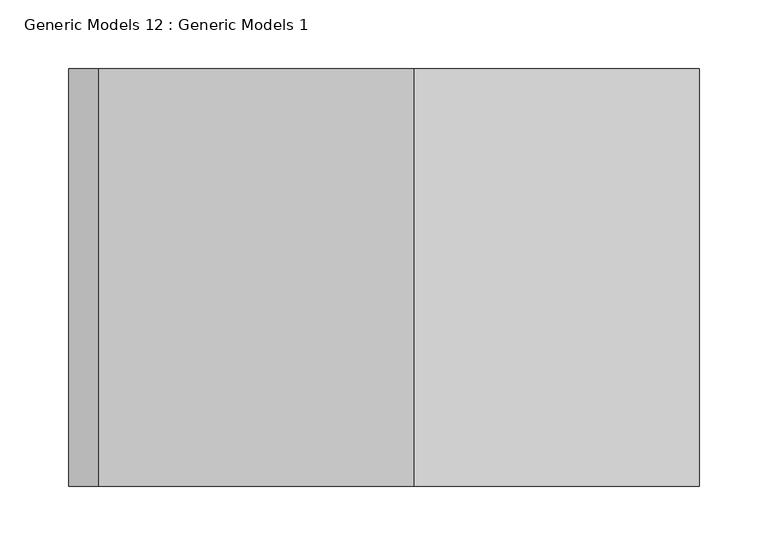
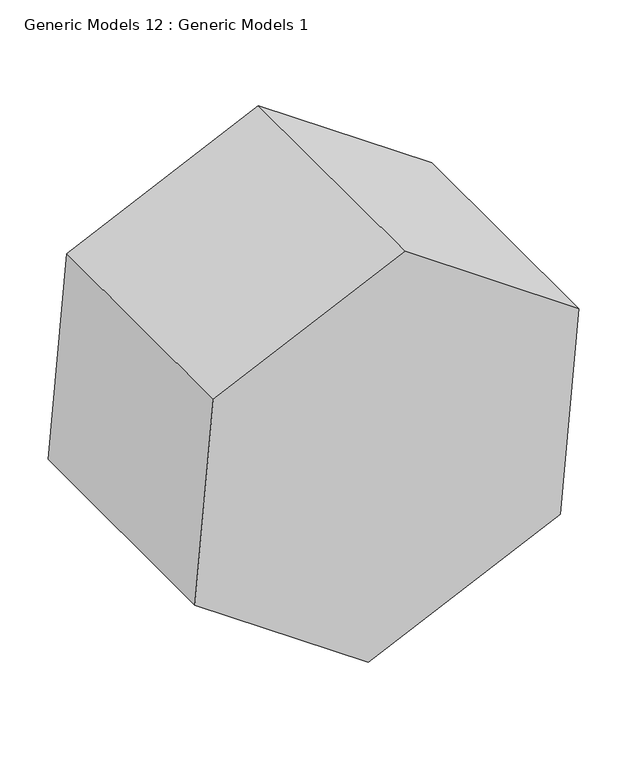
"""IFC4 building model written with IfcOpenShell, lengths in millimetres: proxy geometry, Generic Models 12 : Generic Models 1."""

from ifc_helpers import new_model, si_unit, frame, origin, place, context, project, spatial, polyline, outline, extrude, source, transform, mapped, element, save


def generic_models_12_generic_models_1_297bb3a6(model_context):
    return source(origin(), model_context, "Body", "SweptSolid", [
        extrude(outline(polyline([(833.1013393, 3247.6920945), (978.7897542, 3039.6274753), (871.4447157, 2809.4252974), (618.4112624, 2787.2877387), (472.7228475, 2995.352358), (580.067886, 3225.5545359), (833.1013393, 3247.6920945)])), frame((0.0, -10720.3372434, 0.0), z_axis=(0.0, 1.0, 0.0), x_axis=(0.0, 0.0, 1.0)), (0.0, 0.0, 1.0), 304.8),
    ])


if __name__ == "__main__":
    model = new_model("IFC4")
    model_context = context("Model", 3, world=origin())
    ifc_project = project(units=[si_unit("LENGTHUNIT", "METRE", prefix="MILLI")], contexts=[model_context])
    site = spatial("IfcSite", under=ifc_project)
    building = spatial("IfcBuilding", under=site)
    placement = place(None, origin())
    generic_models_12_generic_models_1_shape = generic_models_12_generic_models_1_297bb3a6(model_context)
    element("IfcBuildingElementProxy", 1, Name="Generic Models 12 : Generic Models 1", ObjectType="Generic Models 12 : Generic Models 1", at=placement, inside=building, context=model_context, shape_type="MappedRepresentation", body=[
        mapped(generic_models_12_generic_models_1_shape, transform((0.0, 0.0, 0.0), x_axis=(1.0, 0.0, 0.0), y_axis=(0.0, 1.0, 0.0), z_axis=(0.0, 0.0, 1.0))),
    ])
    save(model, "model.ifc")

# Revit data of these elements
# Element 1 (IfcBuildingElementProxy, "Generic Models 12 : Generic Models 1")
#   Materials on its faces: "Carpet (1)"
# Materials
#   "Carpet (1)": class "Carpet", colour RGB 124 80 67, transparency 0, Description = "Interior finish", Cost = 0
